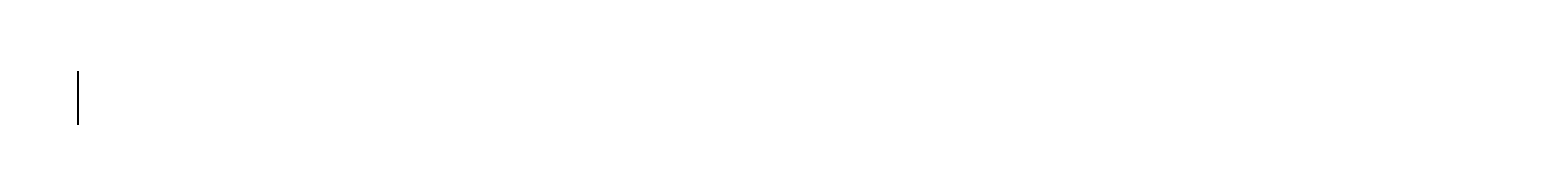
# Model space of a CAD drawing. Units: inches. Extents: x 35362 to 73946, y 43607 to 67532.
# Tile 100 of 134: x 50119 to 50761, y 49298 to 49313. Entities that reach past the tile are written whole.
import ezdxf

# ---------------------------------------------------------------- set-up
doc = ezdxf.new("R2010")
doc.units = ezdxf.units.IN
doc.header["$MEASUREMENT"] = 0
doc.layers.add('A-ANNO-DIMS', color=2, linetype='Continuous', lineweight=18)
doc.styles.get("Standard").update_dxf_attribs({"font": 'arial.ttf'})
doc.dimstyles.get("Standard").update_dxf_attribs({"dimtxt": 0.18, "dimasz": 0.18, "dimexe": 0.18, "dimexo": 0.0625, "dimgap": 0.09, "dimtad": 0, "dimtih": 1, "dimtoh": 1, "dimdec": 4, "dimzin": 0, "dimdsep": 46, "dimtxsty": 'Standard', "dimcen": 0.09, "dimadec": 0, "dimazin": 0, "dimtfac": 1, "dimtdec": 4, "dimtofl": 0, "dimtmove": 0, "dimatfit": 3, "dimfxl": 1, "dimtolj": 1, "dimtzin": 0, "dimarcsym": 0})

# ---------------------------------------------------------------- blocks, each defined once
blk = doc.blocks.new('*D11')
at = {"layer": 'A-ANNO-DIMS', "color": 0, "lineweight": -2, "transparency": 16777216}
for p, q in [((47978.66, 56028.77), (47978.66, 43606.68)), ((53109.76, 56028.77), (53109.76, 43606.68)), ((47978.84, 43606.86), (50543.87, 43606.86)), ((53109.58, 43606.86), (50544.55, 43606.86))]:
    blk.add_line(p, q, dxfattribs=at)
at = {"layer": 'A-ANNO-DIMS', "color": 0, "transparency": 16777216}
for points in [[(47978.84, 43606.89), (47978.84, 43606.83), (47978.66, 43606.86)], [(53109.58, 43606.89), (53109.58, 43606.83), (53109.76, 43606.86)]]:
    blk.add_solid(points, dxfattribs=at)
at = {"layer": 'Defpoints', "color": 0, "transparency": 16777216}
for p in [(47978.66, 56028.84), (53109.76, 56028.84), (53109.76, 43606.86)]:
    blk.add_point(p, dxfattribs=at)
at = {"layer": 'A-ANNO-DIMS', "color": 0, "transparency": 16777216, "insert": (50544.21, 43606.86), "char_height": 0.18, "attachment_point": 5}
blk.add_mtext('\\A1;5131', dxfattribs=at)
blk = doc.blocks.new('*D13')
at = {"layer": 'A-ANNO-DIMS', "color": 0, "lineweight": -2, "transparency": 16777216}
for p, q in [((48373.49, 51694.02), (48373.49, 43606.68)), ((51029.04, 51694.02), (51029.04, 43606.68)), ((48373.67, 43606.86), (49700.8, 43606.86)), ((51028.86, 43606.86), (49701.73, 43606.86))]:
    blk.add_line(p, q, dxfattribs=at)
at = {"layer": 'A-ANNO-DIMS', "color": 0, "transparency": 16777216}
for points in [[(48373.67, 43606.89), (48373.67, 43606.83), (48373.49, 43606.86)], [(51028.86, 43606.89), (51028.86, 43606.83), (51029.04, 43606.86)]]:
    blk.add_solid(points, dxfattribs=at)
at = {"layer": 'Defpoints', "color": 0, "transparency": 16777216}
for p in [(48373.49, 51694.09), (51029.04, 51694.09), (51029.04, 43606.86)]:
    blk.add_point(p, dxfattribs=at)
at = {"layer": 'A-ANNO-DIMS', "color": 0, "transparency": 16777216, "insert": (49701.27, 43606.86), "char_height": 0.18, "attachment_point": 5}
blk.add_mtext('\\A1;2655.6', dxfattribs=at)
blk = doc.blocks.new('*D17')
at = {"layer": 'A-ANNO-DIMS', "color": 0, "lineweight": -2, "transparency": 16777216}
for p, q in [((49923.31, 61293.22), (49923.31, 43606.68)), ((51913.93, 61293.22), (51913.93, 43606.68)), ((49923.49, 43606.86), (50918.16, 43606.86)), ((51913.75, 43606.86), (50919.07, 43606.86))]:
    blk.add_line(p, q, dxfattribs=at)
at = {"layer": 'A-ANNO-DIMS', "color": 0, "transparency": 16777216}
for points in [[(49923.49, 43606.89), (49923.49, 43606.83), (49923.31, 43606.86)], [(51913.75, 43606.89), (51913.75, 43606.83), (51913.93, 43606.86)]]:
    blk.add_solid(points, dxfattribs=at)
at = {"layer": 'Defpoints', "color": 0, "transparency": 16777216}
for p in [(49923.31, 61293.29), (51913.93, 61293.29), (51913.93, 43606.86)]:
    blk.add_point(p, dxfattribs=at)
at = {"layer": 'A-ANNO-DIMS', "color": 0, "transparency": 16777216, "insert": (50918.62, 43606.86), "char_height": 0.18, "attachment_point": 5}
blk.add_mtext('\\A1;1990.6', dxfattribs=at)
blk = doc.blocks.new('*D67')
at = {"layer": 'A-ANNO-DIMS', "color": 0, "lineweight": -2, "transparency": 16777216}
for p, q in [((56873.54, 53351.53), (35361.77, 53351.53)), ((35361.95, 53351.35), (35361.95, 49400.89)), ((35361.95, 45450.07), (35361.95, 49400.53)), ((53793.58, 45449.89), (35361.77, 45449.89))]:
    blk.add_line(p, q, dxfattribs=at)
at = {"layer": 'A-ANNO-DIMS', "color": 0, "transparency": 16777216}
for points in [[(35361.92, 53351.35), (35361.98, 53351.35), (35361.95, 53351.53)], [(35361.92, 45450.07), (35361.98, 45450.07), (35361.95, 45449.89)]]:
    blk.add_solid(points, dxfattribs=at)
at = {"layer": 'Defpoints', "color": 0, "transparency": 16777216}
for p in [(35361.95, 53351.53), (56873.6, 53351.53), (53793.64, 45449.89)]:
    blk.add_point(p, dxfattribs=at)
at = {"layer": 'A-ANNO-DIMS', "color": 0, "transparency": 16777216, "insert": (35361.95, 49400.71), "char_height": 0.18, "attachment_point": 5}
blk.add_mtext('\\A1;7901.6', dxfattribs=at)
blk = doc.blocks.new('*D86')
at = {"layer": 'A-ANNO-DIMS', "color": 0, "lineweight": -2, "transparency": 16777216}
for p, q in [((51285.53, 49320.08), (35361.77, 49320.08)), ((35361.95, 49319.9), (35361.95, 49120.26)), ((35361.95, 48920.26), (35361.95, 49119.9)), ((51285.53, 48920.08), (35361.77, 48920.08))]:
    blk.add_line(p, q, dxfattribs=at)
at = {"layer": 'A-ANNO-DIMS', "color": 0, "transparency": 16777216}
for points in [[(35361.92, 49319.9), (35361.98, 49319.9), (35361.95, 49320.08)], [(35361.92, 48920.26), (35361.98, 48920.26), (35361.95, 48920.08)]]:
    blk.add_solid(points, dxfattribs=at)
at = {"layer": 'Defpoints', "color": 0, "transparency": 16777216}
for p in [(35361.95, 49320.08), (51285.59, 49320.08), (51285.59, 48920.08)]:
    blk.add_point(p, dxfattribs=at)
at = {"layer": 'A-ANNO-DIMS', "color": 0, "transparency": 16777216, "insert": (35361.95, 49120.08), "char_height": 0.18, "attachment_point": 5}
blk.add_mtext('\\A1;400.0', dxfattribs=at)
blk = doc.blocks.new('*D107')
at = {"layer": 'A-ANNO-DIMS', "color": 0, "lineweight": -2, "transparency": 16777216}
for p, q in [((50139.56, 59850.01), (50139.56, 43606.68)), ((51320.81, 59850.01), (51320.81, 43606.68)), ((50139.74, 43606.86), (50729.73, 43606.86)), ((51320.63, 43606.86), (50730.64, 43606.86))]:
    blk.add_line(p, q, dxfattribs=at)
at = {"layer": 'A-ANNO-DIMS', "color": 0, "transparency": 16777216}
for points in [[(50139.74, 43606.89), (50139.74, 43606.83), (50139.56, 43606.86)], [(51320.63, 43606.89), (51320.63, 43606.83), (51320.81, 43606.86)]]:
    blk.add_solid(points, dxfattribs=at)
at = {"layer": 'Defpoints', "color": 0, "transparency": 16777216}
for p in [(50139.56, 59850.08), (51320.81, 59850.08), (51320.81, 43606.86)]:
    blk.add_point(p, dxfattribs=at)
at = {"layer": 'A-ANNO-DIMS', "color": 0, "transparency": 16777216, "insert": (50730.19, 43606.86), "char_height": 0.18, "attachment_point": 5}
blk.add_mtext('\\A1;1181.3', dxfattribs=at)

msp = doc.modelspace()

# ---------------------------------------------------------------- dimensions: what is measured, and where the dimension line sits
at = {"layer": 'A-ANNO-DIMS'}
for base, p1, p2, override, picture, middle in [((51913.931, 43606.859), (49923.307, 61293.286), (51913.931, 61293.286), {"dimdec": 1, "dimlfac": 1, "dimrnd": 0, "dimzin": 0, "dimdsep": 46, "dimlunit": 2}, '*D17', (50918.619, 43606.859)), ((51320.8133, 43606.859), (50139.5627, 59850.0769), (51320.8133, 59850.0769), {"dimdec": 1, "dimlfac": 1, "dimrnd": 0, "dimzin": 0, "dimdsep": 46, "dimlunit": 2}, '*D107', (50730.188, 43606.859)), ((53109.76, 43606.859), (47978.665, 56028.836), (53109.76, 56028.836), {"dimdec": 0, "dimlfac": 1, "dimrnd": 0, "dimzin": 0, "dimdsep": 46, "dimlunit": 2}, '*D11', (50544.212, 43606.859)), ((51029.043, 43606.859), (48373.492, 51694.087), (51029.043, 51694.087), {"dimdec": 1, "dimlfac": 1, "dimrnd": 0, "dimzin": 0, "dimdsep": 46, "dimlunit": 2}, '*D13', (49701.267, 43606.859))]:
    dim = msp.add_linear_dim(base=base, p1=p1, p2=p2, dimstyle='Standard', override=override, dxfattribs=at)
    dim.commit()
    dim.dimension.update_dxf_attribs({"geometry": picture, "text_midpoint": middle})
for base, p1, p2, picture, middle in [((35361.949, 53351.529), (53793.638, 45449.894), (56873.602, 53351.529), '*D67', (35361.949, 49400.712)), ((35361.949, 49320.079), (51285.595, 48920.079), (51285.595, 49320.079), '*D86', (35361.949, 49120.079))]:
    dim = msp.add_linear_dim(base=base, p1=p1, p2=p2, angle=90, dimstyle='Standard', override={"dimdec": 1, "dimlfac": 1, "dimrnd": 0, "dimzin": 0, "dimdsep": 46, "dimlunit": 2}, dxfattribs=at)
    dim.commit()
    dim.dimension.update_dxf_attribs({"geometry": picture, "text_midpoint": middle})

doc.saveas('drawing.dxf')
